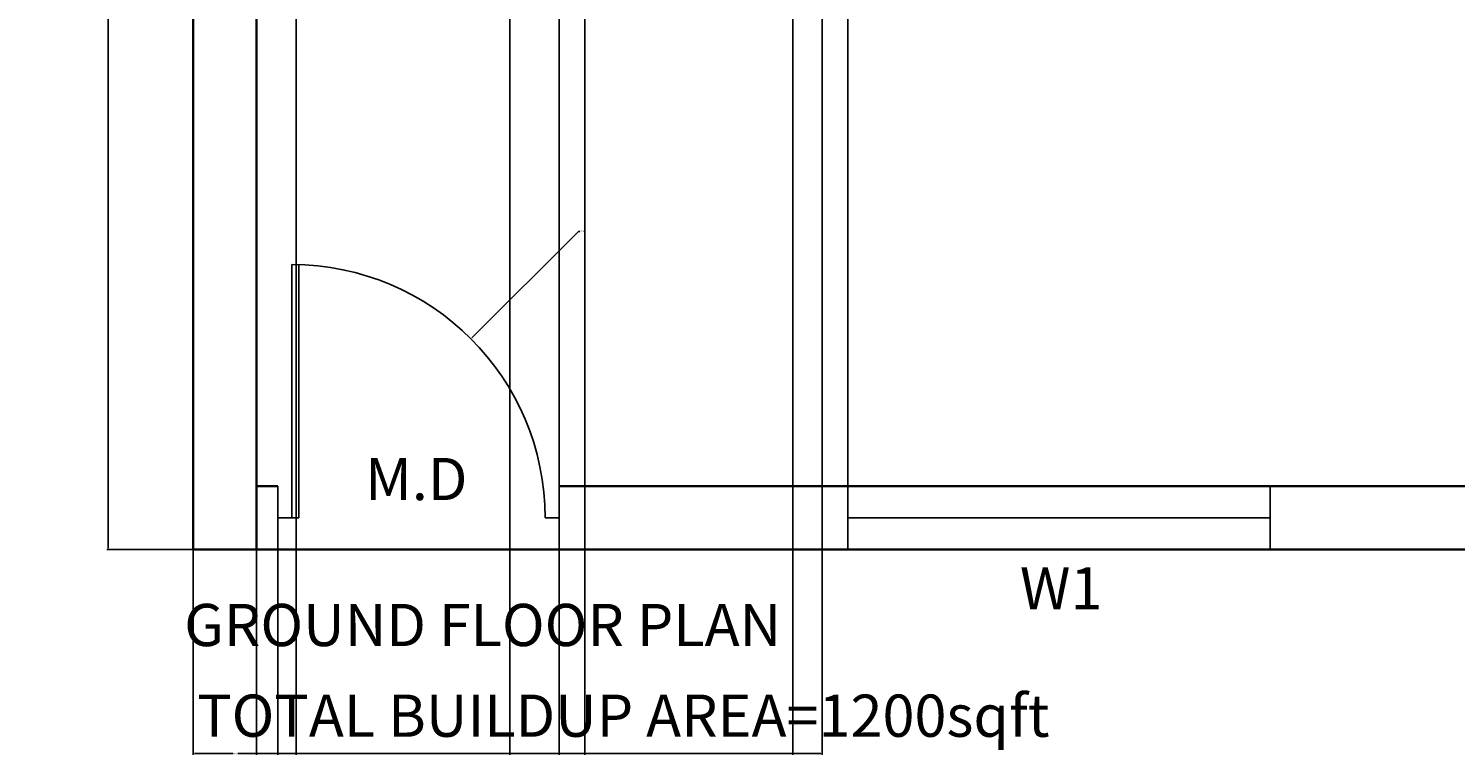
# Model space of a CAD drawing. Units: inches. Extents: x 3 to 420, y -502 to 54.
# Tile 1 of 6: x 9 to 212, y -502 to -398. Entities that reach past the tile are written whole.
import ezdxf

# ---------------------------------------------------------------- set-up
doc = ezdxf.new("R2010")
doc.units = ezdxf.units.IN
doc.header["$MEASUREMENT"] = 0
for name, color, linetype, lineweight in [('A-ANNO-DIMS', 2, 'Continuous', 18), ('A-ANNO-TEXT', 7, 'Continuous', 18), ('A-DOOR', 4, 'Continuous', 25), ('A-GLAZ', 40, 'Continuous', 25), ('A-WALL', 7, 'Continuous', 35)]:
    doc.layers.add(name, color=color, linetype=linetype, lineweight=lineweight)
doc.styles.get("Standard").update_dxf_attribs({"font": 'arial.ttf'})
doc.dimstyles.get("Standard").update_dxf_attribs({"dimtxt": 0.18, "dimasz": 0.18, "dimexe": 0.18, "dimexo": 0.0625, "dimgap": 0.09, "dimtad": 0, "dimtih": 1, "dimtoh": 1, "dimdec": 0, "dimzin": 0, "dimdsep": 46, "dimlunit": 3, "dimtxsty": 'Standard', "dimcen": 0.09, "dimadec": 0, "dimazin": 0, "dimtfac": 1, "dimtdec": 0, "dimtofl": 0, "dimtmove": 0, "dimatfit": 3, "dimfxl": 1, "dimtolj": 1, "dimtzin": 0, "dimarcsym": 0})

# ---------------------------------------------------------------- blocks, each defined once
blk = doc.blocks.new('*D2')
at = {"layer": 'A-ANNO-DIMS', "color": 0, "lineweight": -2, "transparency": 16777216}
for p, q in [((32.33, 4.54), (20.1, 4.54)), ((20.28, 4.36), (20.28, -230.8)), ((20.28, -472.28), (20.28, -237.11)), ((32.33, -472.46), (20.1, -472.46))]:
    blk.add_line(p, q, dxfattribs=at)
at = {"layer": 'A-ANNO-DIMS', "color": 0, "transparency": 16777216}
for points in [[(20.25, 4.36), (20.31, 4.36), (20.28, 4.54)], [(20.25, -472.28), (20.31, -472.28), (20.28, -472.46)]]:
    blk.add_solid(points, dxfattribs=at)
at = {"layer": 'Defpoints', "color": 0, "transparency": 16777216}
for p in [(32.39, 4.54), (20.28, -472.46), (32.39, -472.46)]:
    blk.add_point(p, dxfattribs=at)
at = {"layer": 'A-ANNO-DIMS', "color": 0, "transparency": 16777216, "insert": (20.28, -233.96), "char_height": 6, "attachment_point": 5}
blk.add_mtext('\\A1;39\'-9"', dxfattribs=at)
blk = doc.blocks.new('WIN-W1-60')
for p, q in [((0, 9), (60, 9)), ((0, 9), (0, 0)), ((60, 9), (60, 0)), ((0, 4.5), (60, 4.5)), ((0, 0), (60, 0))]:
    blk.add_line(p, q)
blk = doc.blocks.new('*D39')
at = {"layer": 'A-ANNO-DIMS', "color": 0, "lineweight": -2, "transparency": 16777216}
for p, q in [((41.39, -130.52), (41.39, -501.64)), ((77.36, -130.52), (77.36, -501.64)), ((41.57, -501.46), (59.04, -501.46)), ((77.18, -501.46), (59.7, -501.46))]:
    blk.add_line(p, q, dxfattribs=at)
at = {"layer": 'A-ANNO-DIMS', "color": 0, "transparency": 16777216}
for points in [[(41.57, -501.43), (41.57, -501.49), (41.39, -501.46)], [(77.18, -501.43), (77.18, -501.49), (77.36, -501.46)]]:
    blk.add_solid(points, dxfattribs=at)
at = {"layer": 'Defpoints', "color": 0, "transparency": 16777216}
for p in [(41.39, -130.46), (77.36, -130.46), (77.36, -501.46)]:
    blk.add_point(p, dxfattribs=at)
at = {"layer": 'A-ANNO-DIMS', "color": 0, "transparency": 16777216, "insert": (59.37, -501.46), "char_height": 0.18, "attachment_point": 5}
blk.add_mtext('\\A1;3\'-0"', dxfattribs=at)
blk = doc.blocks.new('*D46')
at = {"layer": 'A-ANNO-DIMS', "color": 0, "lineweight": -2, "transparency": 16777216}
for p, q in [((41.39, -135.02), (41.39, -501.64)), ((121.75, -135.02), (121.75, -501.64)), ((41.57, -501.46), (81.03, -501.46)), ((121.57, -501.46), (82.11, -501.46))]:
    blk.add_line(p, q, dxfattribs=at)
at = {"layer": 'A-ANNO-DIMS', "color": 0, "transparency": 16777216}
for points in [[(41.57, -501.43), (41.57, -501.49), (41.39, -501.46)], [(121.57, -501.43), (121.57, -501.49), (121.75, -501.46)]]:
    blk.add_solid(points, dxfattribs=at)
at = {"layer": 'Defpoints', "color": 0, "transparency": 16777216}
for p in [(41.39, -134.96), (121.75, -134.96), (121.75, -501.46)]:
    blk.add_point(p, dxfattribs=at)
at = {"layer": 'A-ANNO-DIMS', "color": 0, "transparency": 16777216, "insert": (81.57, -501.46), "char_height": 0.18, "attachment_point": 5}
blk.add_mtext('\\A1;6\'-8 1/2"', dxfattribs=at)
blk = doc.blocks.new('*D50')
at = {"layer": 'A-ANNO-DIMS', "color": 0, "lineweight": -2, "transparency": 16777216}
for p, q in [((44.39, -472.52), (44.39, -501.64)), ((84.39, -472.52), (84.39, -501.64)), ((44.57, -501.46), (64.06, -501.46)), ((84.21, -501.46), (64.72, -501.46))]:
    blk.add_line(p, q, dxfattribs=at)
at = {"layer": 'A-ANNO-DIMS', "color": 0, "transparency": 16777216}
for points in [[(44.57, -501.43), (44.57, -501.49), (44.39, -501.46)], [(84.21, -501.43), (84.21, -501.49), (84.39, -501.46)]]:
    blk.add_solid(points, dxfattribs=at)
at = {"layer": 'Defpoints', "color": 0, "transparency": 16777216}
for p in [(44.39, -472.46), (84.39, -472.46), (84.39, -501.46)]:
    blk.add_point(p, dxfattribs=at)
at = {"layer": 'A-ANNO-DIMS', "color": 0, "transparency": 16777216, "insert": (64.39, -501.46), "char_height": 0.18, "attachment_point": 5}
blk.add_mtext('\\A1;3\'-4"', dxfattribs=at)
blk = doc.blocks.new('*D62')
at = {"layer": 'A-ANNO-DIMS', "color": 0, "lineweight": -2, "transparency": 16777216}
for p, q in [((84.39, -463.39), (84.39, 33.72)), ((84.57, 33.54), (104.58, 33.54)), ((125.25, 33.54), (105.24, 33.54)), ((125.43, -463.39), (125.43, 33.72))]:
    blk.add_line(p, q, dxfattribs=at)
at = {"layer": 'A-ANNO-DIMS', "color": 0, "transparency": 16777216}
for points in [[(84.57, 33.57), (84.57, 33.51), (84.39, 33.54)], [(125.25, 33.57), (125.25, 33.51), (125.43, 33.54)]]:
    blk.add_solid(points, dxfattribs=at)
at = {"layer": 'Defpoints', "color": 0, "transparency": 16777216}
for p in [(125.43, 33.54), (84.39, -463.46), (125.43, -463.46)]:
    blk.add_point(p, dxfattribs=at)
at = {"layer": 'A-ANNO-DIMS', "color": 0, "transparency": 16777216, "insert": (104.91, 33.54), "char_height": 0.18, "attachment_point": 5}
blk.add_mtext('\\A1;3\'-5"', dxfattribs=at)
blk = doc.blocks.new('*D63')
at = {"layer": 'A-ANNO-DIMS', "color": 0, "lineweight": -2, "transparency": 16777216}
for p, q in [((32.39, -472.52), (32.39, -501.64)), ((44.39, -472.52), (44.39, -501.64)), ((32.57, -501.46), (38.07, -501.46)), ((44.21, -501.46), (38.71, -501.46))]:
    blk.add_line(p, q, dxfattribs=at)
at = {"layer": 'A-ANNO-DIMS', "color": 0, "transparency": 16777216}
for points in [[(32.57, -501.43), (32.57, -501.49), (32.39, -501.46)], [(44.21, -501.43), (44.21, -501.49), (44.39, -501.46)]]:
    blk.add_solid(points, dxfattribs=at)
at = {"layer": 'Defpoints', "color": 0, "transparency": 16777216}
for p in [(32.39, -472.46), (44.39, -472.46), (44.39, -501.46)]:
    blk.add_point(p, dxfattribs=at)
at = {"layer": 'A-ANNO-DIMS', "color": 0, "transparency": 16777216, "insert": (38.39, -501.46), "char_height": 0.18, "attachment_point": 5}
blk.add_mtext('\\A1;1\'-0"', dxfattribs=at)
blk = doc.blocks.new('*D73')
at = {"layer": 'A-ANNO-DIMS', "color": 0, "lineweight": -2, "transparency": 16777216}
for p, q in [((88.02, -313.52), (88.02, -501.64)), ((117.58, -313.52), (117.58, -501.64)), ((88.2, -501.46), (102.26, -501.46)), ((117.4, -501.46), (103.34, -501.46))]:
    blk.add_line(p, q, dxfattribs=at)
at = {"layer": 'A-ANNO-DIMS', "color": 0, "transparency": 16777216}
for points in [[(88.2, -501.43), (88.2, -501.49), (88.02, -501.46)], [(117.4, -501.43), (117.4, -501.49), (117.58, -501.46)]]:
    blk.add_solid(points, dxfattribs=at)
at = {"layer": 'Defpoints', "color": 0, "transparency": 16777216}
for p in [(88.02, -313.46), (117.58, -313.46), (117.58, -501.46)]:
    blk.add_point(p, dxfattribs=at)
at = {"layer": 'A-ANNO-DIMS', "color": 0, "transparency": 16777216, "insert": (102.8, -501.46), "char_height": 0.18, "attachment_point": 5}
blk.add_mtext('\\A1;2\'-5 1/2"', dxfattribs=at)
blk = doc.blocks.new('*D78')
at = {"layer": 'A-ANNO-DIMS', "color": 0, "lineweight": -2, "transparency": 16777216}
for p, q in [((46.99, -331.21), (46.99, -501.64)), ((41.39, -336.02), (41.39, -501.64)), ((41.57, -501.46), (43.65, -501.46)), ((46.81, -501.46), (44.73, -501.46))]:
    blk.add_line(p, q, dxfattribs=at)
at = {"layer": 'A-ANNO-DIMS', "color": 0, "transparency": 16777216}
for points in [[(41.57, -501.43), (41.57, -501.49), (41.39, -501.46)], [(46.81, -501.43), (46.81, -501.49), (46.99, -501.46)]]:
    blk.add_solid(points, dxfattribs=at)
at = {"layer": 'Defpoints', "color": 0, "transparency": 16777216}
for p in [(46.99, -331.15), (41.39, -335.96), (46.99, -501.46)]:
    blk.add_point(p, dxfattribs=at)
at = {"layer": 'A-ANNO-DIMS', "color": 0, "transparency": 16777216, "insert": (44.19, -501.46), "char_height": 0.18, "attachment_point": 5}
blk.add_mtext('\\A1;0\'-5 1/2"', dxfattribs=at)
blk = doc.blocks.new('*D83')
at = {"layer": 'A-ANNO-DIMS', "color": 0, "lineweight": -2, "transparency": 16777216}
for p, q in [((87.12, -427.23), (71.97, -442.37)), ((87.3, -427.23), (87.12, -427.23)), ((46.3, -467.96), (46.48, -467.96)), ((46.39, -468.05), (46.39, -467.87))]:
    blk.add_line(p, q, dxfattribs=at)
at = {"layer": 'A-ANNO-DIMS', "color": 0, "transparency": 16777216}
blk.add_solid([(71.95, -442.35), (71.99, -442.39), (71.84, -442.5)], dxfattribs=at)
at = {"layer": 'Defpoints', "color": 0, "transparency": 16777216}
for p in [(71.84, -442.5), (46.39, -467.96)]:
    blk.add_point(p, dxfattribs=at)
at = {"layer": 'A-ANNO-DIMS', "color": 0, "transparency": 16777216, "insert": (87.71, -427.23), "char_height": 0.18, "attachment_point": 5}
blk.add_mtext('\\A1;R3\'-0"', dxfattribs=at)

msp = doc.modelspace()

# ---------------------------------------------------------------- linework, layer by layer
at = {"layer": 'A-DOOR'}
for p, q in [((46.39, -467.96), (46.39, -431.96)), ((47.39, -467.96), (47.39, -431.96)), ((44.39, -463.46), (44.39, -472.46)), ((84.39, -467.96), (84.39, -463.46)), ((44.39, -467.96), (46.39, -467.96)), ((46.39, -467.96), (47.39, -467.96)), ((82.39, -467.96), (84.39, -467.96)), ((84.39, -467.96), (84.39, -472.46))]:
    msp.add_line(p, q, dxfattribs=at)
msp.add_arc((46.39, -467.96), 36, 0, 90, dxfattribs=at)
at = {"layer": 'A-WALL'}
for p, q in [((32.39, 4.54), (32.39, -472.46)), ((41.39, -259.46), (41.39, -472.46)), ((41.39, -463.46), (44.39, -463.46)), ((84.39, -463.46), (381.89, -463.46)), ((32.39, -472.46), (390.89, -472.46))]:
    msp.add_line(p, q, dxfattribs=at)

# ---------------------------------------------------------------- block references
at = {"layer": 'A-GLAZ'}
msp.add_blockref('WIN-W1-60', (125.43, -472.46), dxfattribs=at)

# ---------------------------------------------------------------- texts
at = {"layer": 'A-ANNO-TEXT', "char_height": 6, "attachment_point": 1}
for s, insert in [('M.D', (56.8, -459.43)), ('W1', (149.86, -474.97)), ('GROUND FLOOR PLAN', (31.09, -480.18)), ('TOTAL BUILDUP AREA=1200sqft', (32.93, -493.07))]:
    msp.add_mtext(s, dxfattribs=dict(at, insert=insert))

# ---------------------------------------------------------------- dimensions: what is measured, and where the dimension line sits
at = {"layer": 'A-ANNO-DIMS'}
for base, p1, p2, picture, middle in [((125.43, 33.54), (84.39, -463.46), (125.43, -463.46), '*D62', (104.91, 33.54)), ((77.36, -501.46), (41.39, -130.46), (77.36, -130.46), '*D39', (59.37, -501.46)), ((121.75, -501.46), (41.39, -134.96), (121.75, -134.96), '*D46', (81.57, -501.46)), ((117.58, -501.46), (88.02, -313.46), (117.58, -313.46), '*D73', (102.8, -501.46)), ((46.99, -501.46), (41.39, -335.96), (46.99, -331.15), '*D78', (44.19, -501.46)), ((44.39, -501.46), (32.39, -472.46), (44.39, -472.46), '*D63', (38.39, -501.46)), ((84.39, -501.46), (44.39, -472.46), (84.39, -472.46), '*D50', (64.39, -501.46))]:
    dim = msp.add_linear_dim(base=base, p1=p1, p2=p2, dimstyle='Standard', override={"dimdec": 1, "dimlfac": 1, "dimrnd": 0, "dimzin": 1, "dimdsep": 46, "dimlunit": 4, "dimfrac": 2}, dxfattribs=at)
    dim.commit()
    dim.dimension.update_dxf_attribs({"geometry": picture, "text_midpoint": middle})
dim = msp.add_linear_dim(base=(20.28, -472.46), p1=(32.39, 4.54), p2=(32.39, -472.46), angle=90, dimstyle='Standard', override={"dimtxt": 6, "dimclrd": 0, "dimclre": 0, "dimclrt": 0}, dxfattribs=at)
dim.commit()
dim.dimension.update_dxf_attribs({"geometry": '*D2', "text_midpoint": (20.28, -233.96)})
dim = msp.add_radius_dim(center=(46.39, -467.96), mpoint=(71.84, -442.5), dimstyle='Standard', override={"dimdec": 1, "dimlfac": 1, "dimrnd": 0, "dimzin": 1, "dimdsep": 46, "dimlunit": 4, "dimfrac": 2}, dxfattribs=at)
dim.commit()
dim.dimension.update_dxf_attribs({"geometry": '*D83', "text_midpoint": (87.71, -427.23), "dimtype": 164})

doc.saveas('drawing.dxf')
